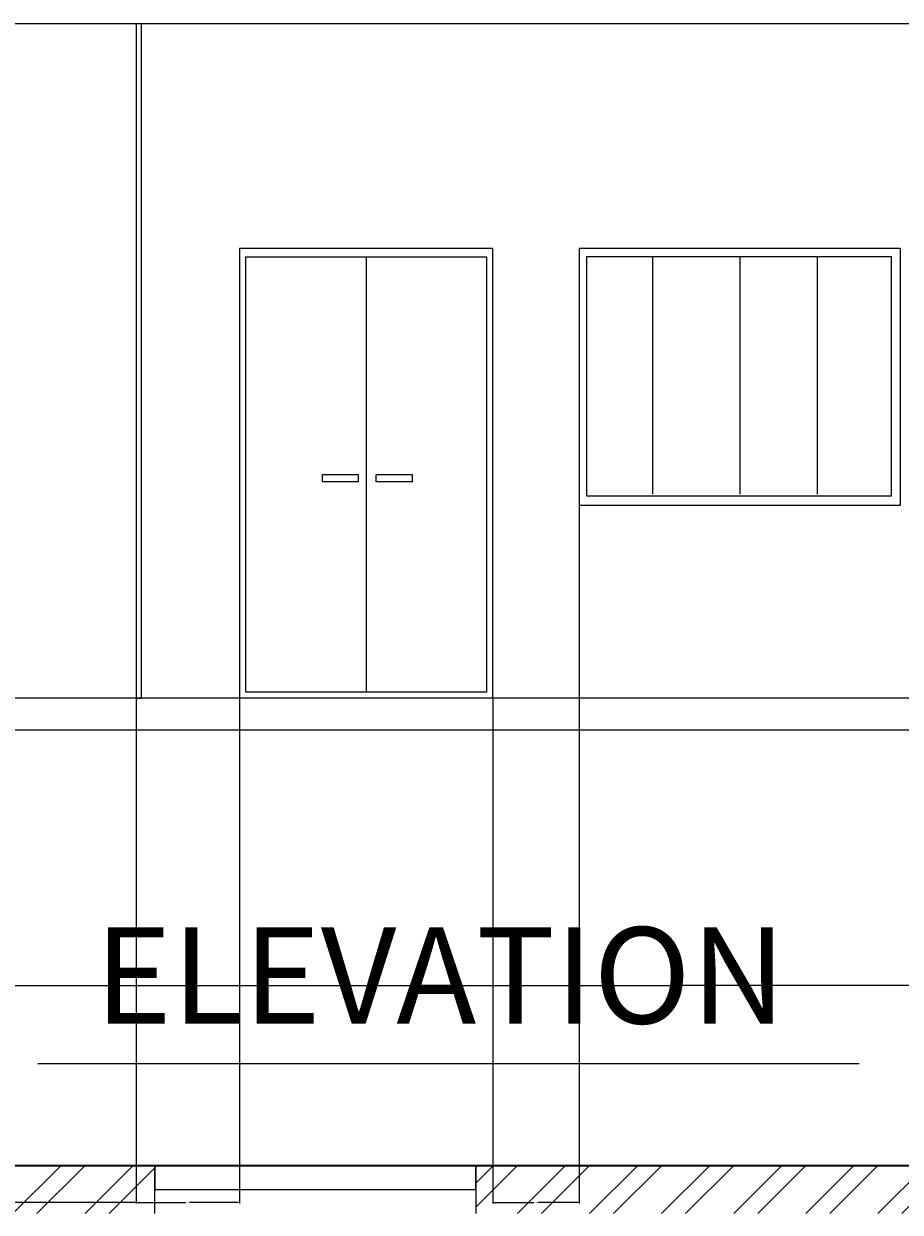
# Model space of a CAD drawing. Units: inches. Extents: x 1152 to 2588, y 1459 to 2618.
# Tile 12 of 17: x 1384 to 1548, y 2231 to 2453. Entities that reach past the tile are written whole.
import ezdxf

# ---------------------------------------------------------------- set-up
doc = ezdxf.new("R2010")
doc.units = ezdxf.units.IN
for name, color, linetype, lineweight in [('A-ANNO-DIMS', 2, 'Continuous', 18), ('A-ANNO-TEXT', 7, 'Continuous', 18), ('A-DOOR', 4, 'Continuous', 18), ('A-ELEV', 7, 'Continuous', 25), ('A-GLAZ', 4, 'Continuous', 18), ('A-WALL', 7, 'Continuous', 35), ('A-WALL-PATT', 8, 'Continuous', 13)]:
    doc.layers.add(name, color=color, linetype=linetype, lineweight=lineweight)
doc.styles.get("Standard").update_dxf_attribs({"font": 'arial.ttf'})
doc.dimstyles.get("Standard").update_dxf_attribs({"dimtxt": 0.18, "dimasz": 0.18, "dimexe": 0.18, "dimexo": 0.0625, "dimgap": 0.09, "dimtad": 0, "dimtih": 1, "dimtoh": 1, "dimdec": 4, "dimzin": 0, "dimdsep": 46, "dimtxsty": 'Standard', "dimcen": 0.09, "dimadec": 0, "dimazin": 0, "dimtfac": 1, "dimtdec": 4, "dimtofl": 0, "dimtmove": 0, "dimatfit": 3, "dimfxl": 1, "dimtolj": 1, "dimtzin": 0, "dimarcsym": 0})

# ---------------------------------------------------------------- blocks, each defined once
blk = doc.blocks.new('WIN-60-BED-NORTH')
for p, q in [((0, 0), (0, 9)), ((0, 9), (0, 4.5)), ((60, 4.5), (60, 9)), ((60, 9), (60, 0)), ((0, 4.5), (60, 4.5))]:
    blk.add_line(p, q)
blk = doc.blocks.new('*D70')
at = {"layer": 'A-ANNO-DIMS', "color": 0, "lineweight": -2, "transparency": 16777216}
for p, q in [((1276.42, 2240.11), (1276.42, 2273.83)), ((1276.6, 2273.65), (1506.12, 2273.65)), ((1736.24, 2273.65), (1506.71, 2273.65)), ((1736.42, 2240.11), (1736.42, 2273.83))]:
    blk.add_line(p, q, dxfattribs=at)
at = {"layer": 'A-ANNO-DIMS', "color": 0, "transparency": 16777216}
for points in [[(1276.6, 2273.68), (1276.6, 2273.62), (1276.42, 2273.65)], [(1736.24, 2273.68), (1736.24, 2273.62), (1736.42, 2273.65)]]:
    blk.add_solid(points, dxfattribs=at)
at = {"layer": 'Defpoints', "color": 0, "transparency": 16777216}
for p in [(1736.42, 2273.65), (1276.42, 2240.05), (1736.42, 2240.05)]:
    blk.add_point(p, dxfattribs=at)
at = {"layer": 'A-ANNO-DIMS', "color": 0, "transparency": 16777216, "insert": (1506.42, 2273.65), "char_height": 0.18, "attachment_point": 5}
blk.add_mtext('\\A1;460', dxfattribs=at)
blk = doc.blocks.new('*D91')
at = {"layer": 'A-ANNO-DIMS', "color": 0, "lineweight": -2, "transparency": 16777216}
for p, q in [((1405.42, 2327.33), (1405.42, 2232.94)), ((1276.42, 2321.33), (1276.42, 2232.94)), ((1276.6, 2233.12), (1340.64, 2233.12)), ((1405.24, 2233.12), (1341.2, 2233.12))]:
    blk.add_line(p, q, dxfattribs=at)
at = {"layer": 'A-ANNO-DIMS', "color": 0, "transparency": 16777216}
for points in [[(1276.6, 2233.15), (1276.6, 2233.09), (1276.42, 2233.12)], [(1405.24, 2233.15), (1405.24, 2233.09), (1405.42, 2233.12)]]:
    blk.add_solid(points, dxfattribs=at)
at = {"layer": 'Defpoints', "color": 0, "transparency": 16777216}
for p in [(1405.42, 2327.39), (1276.42, 2321.39), (1405.42, 2233.12)]:
    blk.add_point(p, dxfattribs=at)
at = {"layer": 'A-ANNO-DIMS', "color": 0, "transparency": 16777216, "insert": (1340.92, 2233.12), "char_height": 0.18, "attachment_point": 5}
blk.add_mtext('\\A1;129', dxfattribs=at)
blk = doc.blocks.new('*D92')
at = {"layer": 'A-ANNO-DIMS', "color": 0, "lineweight": -2, "transparency": 16777216}
for p, q in [((1405.42, 2327.33), (1405.42, 2232.94)), ((1424.73, 2327.33), (1424.73, 2232.94)), ((1405.6, 2233.12), (1414.7, 2233.12)), ((1424.55, 2233.12), (1415.44, 2233.12))]:
    blk.add_line(p, q, dxfattribs=at)
at = {"layer": 'A-ANNO-DIMS', "color": 0, "transparency": 16777216}
for points in [[(1405.6, 2233.15), (1405.6, 2233.09), (1405.42, 2233.12)], [(1424.55, 2233.15), (1424.55, 2233.09), (1424.73, 2233.12)]]:
    blk.add_solid(points, dxfattribs=at)
at = {"layer": 'Defpoints', "color": 0, "transparency": 16777216}
for p in [(1405.42, 2327.39), (1424.73, 2327.39), (1424.73, 2233.12)]:
    blk.add_point(p, dxfattribs=at)
at = {"layer": 'A-ANNO-DIMS', "color": 0, "transparency": 16777216, "insert": (1415.07, 2233.12), "char_height": 0.18, "attachment_point": 5}
blk.add_mtext('\\A1;19.31', dxfattribs=at)
blk = doc.blocks.new('*D93')
at = {"layer": 'A-ANNO-DIMS', "color": 0, "lineweight": -2, "transparency": 16777216}
for p, q in [((1488.24, 2363.33), (1488.24, 2232.94)), ((1472.07, 2327.33), (1472.07, 2232.94)), ((1472.25, 2233.12), (1479.77, 2233.12)), ((1488.06, 2233.12), (1480.54, 2233.12))]:
    blk.add_line(p, q, dxfattribs=at)
at = {"layer": 'A-ANNO-DIMS', "color": 0, "transparency": 16777216}
for points in [[(1472.25, 2233.15), (1472.25, 2233.09), (1472.07, 2233.12)], [(1488.06, 2233.15), (1488.06, 2233.09), (1488.24, 2233.12)]]:
    blk.add_solid(points, dxfattribs=at)
at = {"layer": 'Defpoints', "color": 0, "transparency": 16777216}
for p in [(1488.24, 2363.39), (1472.07, 2327.39), (1488.24, 2233.12)]:
    blk.add_point(p, dxfattribs=at)
at = {"layer": 'A-ANNO-DIMS', "color": 0, "transparency": 16777216, "insert": (1480.15, 2233.12), "char_height": 0.18, "attachment_point": 5}
blk.add_mtext('\\A1;16.17', dxfattribs=at)

msp = doc.modelspace()

# ---------------------------------------------------------------- hatches: boundary and pattern name
at = {"layer": 'A-WALL-PATT'}
h = msp.add_hatch(dxfattribs=at)
h.set_pattern_fill('ANSI32', color=256)
h.paths.add_polyline_path([(1408.9272, 2240.0458), (1276.4165, 2240.0458), (1276.4165, 2192.7491), (1285.4165, 2192.7491), (1285.4165, 2231.0458), (1369.4165, 2231.0458), (1369.4165, 2084.0458), (1526.9165, 2084.0458), (1526.9165, 2096.3728), (1524.6665, 2096.3728), (1522.4165, 2096.3728), (1522.4165, 2093.0458), (1378.4165, 2093.0458), (1378.4165, 2231.0458), (1408.9272, 2231.0458)])
h.paths.add_polyline_path([(1736.4165, 2240.0458), (1468.9272, 2240.0458), (1468.9272, 2231.0458), (1522.4165, 2231.0458), (1522.4165, 2127.3313), (1526.9165, 2127.3313), (1526.9165, 2231.0458), (1574.9165, 2231.0458), (1574.9165, 2188.0458), (1579.4165, 2188.0458), (1579.4165, 2231.0458), (1727.4165, 2231.0458), (1727.4165, 2183.9728), (1736.4165, 2183.9728)])
h.paths.add_polyline_path([(1285.4165, 2156.7491), (1276.4165, 2156.7491), (1276.4165, 2084.0458), (1285.4165, 2084.0458)], flags=17)
h.paths.add_polyline_path([(1285.4165, 2043.5458), (1445.4165, 2043.5458), (1445.4165, 1943.6503), (1454.4165, 1943.6503), (1454.4165, 2048.0458), (1276.4165, 2048.0458), (1276.4165, 2019.2077), (1280.9165, 2019.2077), (1285.4165, 2019.2077)])
h.paths.add_polyline_path([(1285.4165, 1959.2077), (1276.4165, 1959.2077), (1276.4165, 1891.1319), (1280.9165, 1891.1319), (1285.4165, 1891.1319), (1285.4165, 1901.0458), (1376.8505, 1901.0458), (1376.8505, 1903.2958), (1376.8505, 1905.5458), (1285.4165, 1905.5458)])
h.paths.add_polyline_path([(1518.4165, 1905.5458), (1399.2832, 1905.5458), (1399.2832, 1903.2958), (1399.2832, 1901.0458), (1405.4165, 1901.0458), (1405.4165, 1884.8579), (1409.9165, 1884.8579), (1409.9165, 1901.0458), (1513.9165, 1901.0458), (1513.9165, 1869.1706), (1518.4165, 1869.1706)])
h.paths.add_polyline_path([(1520.5229, 1845.0458), (1518.4165, 1845.0458), (1518.4165, 1849.2927), (1516.1665, 1849.2927), (1513.9165, 1849.2927), (1513.9165, 1845.0458), (1409.9165, 1845.0458), (1409.9165, 1860.8579), (1405.4165, 1860.8579), (1405.4165, 1845.0458), (1285.4165, 1845.0458), (1285.4165, 1867.1319), (1276.4165, 1867.1319), (1276.4165, 1635.0458), (1285.4165, 1635.0458), (1285.4165, 1836.0458), (1405.4165, 1836.0458), (1405.4165, 1635.0458), (1414.4165, 1635.0458), (1424.7277, 1635.0458), (1424.7277, 1639.5458), (1424.7277, 1644.0458), (1414.4165, 1644.0458), (1414.4165, 1836.0458), (1414.4165, 1840.5831), (1520.5229, 1840.5831)])
h.paths.add_polyline_path([(1579.4165, 1840.5458), (1583.4035, 1840.5458), (1583.4035, 1845.0458), (1579.4165, 1845.0458), (1570.4165, 1845.0458), (1570.4165, 1840.5831), (1570.4165, 1644.0458), (1548.2359, 1644.0458), (1548.2359, 1635.0458), (1611.2801, 1635.0458), (1611.2801, 1639.5458), (1611.2801, 1644.0458), (1579.4165, 1644.0458)])
h.paths.add_polyline_path([(1488.2359, 1644.0458), (1472.0663, 1644.0458), (1472.0663, 1635.0458), (1488.2359, 1635.0458), (1488.2359, 1639.5458)], flags=17)
h.paths.add_polyline_path([(1736.4165, 1701.1863), (1727.4165, 1701.1863), (1727.4165, 1644.0458), (1671.2801, 1644.0458), (1671.2801, 1635.0458), (1736.4165, 1635.0458)])
h.paths.add_polyline_path([(1736.4165, 2147.9728), (1727.4165, 2147.9728), (1727.4165, 2093.0458), (1579.4165, 2093.0458), (1574.9165, 2093.0458), (1574.9165, 1971.6501), (1579.4165, 1971.6501), (1579.4165, 2084.0458), (1727.4165, 2084.0458), (1727.4165, 2054.3847), (1736.4165, 2054.3847)])
h.paths.add_polyline_path([(1736.4165, 1994.3847), (1727.4165, 1994.3847), (1727.4165, 1911.3562), (1736.4165, 1911.3562)])
h.paths.add_polyline_path([(1736.4165, 1875.3562), (1727.4165, 1875.3562), (1727.4165, 1845.0458), (1617.1767, 1845.0458), (1617.1767, 1842.7958), (1617.1767, 1840.5458), (1618.9165, 1840.5458), (1618.9165, 1788.5458), (1618.9165, 1784.0458), (1627.8699, 1784.0458), (1627.8699, 1788.5458), (1623.4165, 1788.5458), (1623.4165, 1840.5458), (1727.4165, 1840.5458), (1727.4165, 1828.7619), (1736.4165, 1828.7619)])
h.paths.add_polyline_path([(1727.4165, 1938.0458), (1579.4165, 1938.0458), (1579.4165, 1942.7722), (1574.9165, 1942.7722), (1574.9165, 1929.0458), (1727.4165, 1929.0458)])

# ---------------------------------------------------------------- linework, layer by layer
at = {"layer": 'A-ANNO-TEXT'}
msp.add_line((1540.5687, 2259.02), (1387.07, 2259.02), dxfattribs=at)
at = {"layer": 'A-DOOR'}
for p, q in [((1424.7277, 2411.3911), (1424.7277, 2327.3911)), ((1472.0663, 2411.3911), (1424.7277, 2411.3911)), ((1448.4142, 2409.8295), (1448.4142, 2328.4982)), ((1472.0663, 2411.3911), (1472.0663, 2327.3911))]:
    msp.add_line(p, q, dxfattribs=at)
for points in [[(1425.9271, 2409.8295), (1470.9013, 2409.8295), (1470.9013, 2328.4982), (1425.9271, 2328.4982)], [(1440.2512, 2369.1573), (1446.9575, 2369.1573), (1446.9575, 2367.7703), (1440.2512, 2367.7703)], [(1450.3061, 2369.1573), (1457.0124, 2369.1573), (1457.0124, 2367.7703), (1450.3061, 2367.7703)]]:
    msp.add_lwpolyline(points, close=True, dxfattribs=at)
at = {"layer": 'A-ELEV'}
for p, q in [((1760.4165, 2453.3911), (1252.4165, 2453.3911)), ((1405.4165, 2453.3911), (1405.4165, 2327.3911)), ((1406.4165, 2327.3911), (1406.4165, 2453.3911)), ((1736.4165, 2327.3911), (1285.4165, 2327.3911)), ((1405.4165, 2327.3911), (1406.4165, 2327.3911)), ((1736.4165, 2321.3911), (1276.4165, 2321.3911))]:
    msp.add_line(p, q, dxfattribs=at)
at = {"layer": 'A-GLAZ'}
for p, q in [((1488.2359, 2411.3911), (1488.2359, 2363.3911)), ((1548.2359, 2411.3911), (1488.2359, 2411.3911)), ((1501.9211, 2409.8158), (1501.9211, 2365.4866)), ((1518.2359, 2409.8158), (1518.2359, 2365.4866)), ((1532.7322, 2409.8158), (1532.7322, 2365.4866)), ((1548.2359, 2411.3911), (1548.2359, 2363.3911)), ((1548.2359, 2363.3911), (1488.2359, 2363.3911))]:
    msp.add_line(p, q, dxfattribs=at)
msp.add_lwpolyline([(1489.6663, 2409.9035), (1546.5607, 2409.9035), (1546.5607, 2365.1388), (1489.6663, 2365.1388)], close=True, dxfattribs=at)
at = {"layer": 'A-WALL'}
msp.add_line((1276.4165, 2240.0458), (1736.4165, 2240.0458), dxfattribs=at)

# ---------------------------------------------------------------- block references
at = {"layer": 'A-GLAZ'}
msp.add_blockref('WIN-60-BED-NORTH', (1408.927, 2231.046), dxfattribs=at)

# ---------------------------------------------------------------- texts
at = {"layer": 'A-ANNO-TEXT', "insert": (1397.6792, 2284.5603), "char_height": 18, "attachment_point": 1}
msp.add_mtext_dynamic_manual_height_columns('ELEVATION', width=372.313503, gutter_width=12.5, heights=[0], dxfattribs=at)

# ---------------------------------------------------------------- dimensions: what is measured, and where the dimension line sits
at = {"layer": 'A-ANNO-DIMS'}
for base, p1, p2, override, picture, middle in [((1488.2359, 2233.12), (1472.0663, 2327.3911), (1488.2359, 2363.3911), {"dimdec": 2, "dimlfac": 1, "dimrnd": 0, "dimzin": 0, "dimdsep": 46, "dimlunit": 2}, '*D93', (1480.1511, 2233.12)), ((1405.4165, 2233.12), (1276.4165, 2321.3911), (1405.4165, 2327.3911), {"dimdec": 0, "dimlfac": 1, "dimrnd": 0, "dimzin": 0, "dimdsep": 46, "dimlunit": 2}, '*D91', (1340.9165, 2233.12)), ((1424.7277, 2233.12), (1405.4165, 2327.3911), (1424.7277, 2327.3911), {"dimdec": 2, "dimlfac": 1, "dimrnd": 0, "dimzin": 0, "dimdsep": 46, "dimlunit": 2}, '*D92', (1415.0721, 2233.12)), ((1736.4165, 2273.6458), (1276.4165, 2240.0458), (1736.4165, 2240.0458), {"dimdec": 0, "dimlfac": 1, "dimrnd": 0, "dimzin": 0, "dimdsep": 46, "dimlunit": 2}, '*D70', (1506.4165, 2273.6458))]:
    dim = msp.add_linear_dim(base=base, p1=p1, p2=p2, dimstyle='Standard', override=override, dxfattribs=at)
    dim.commit()
    dim.dimension.update_dxf_attribs({"geometry": picture, "text_midpoint": middle})

doc.saveas('drawing.dxf')
